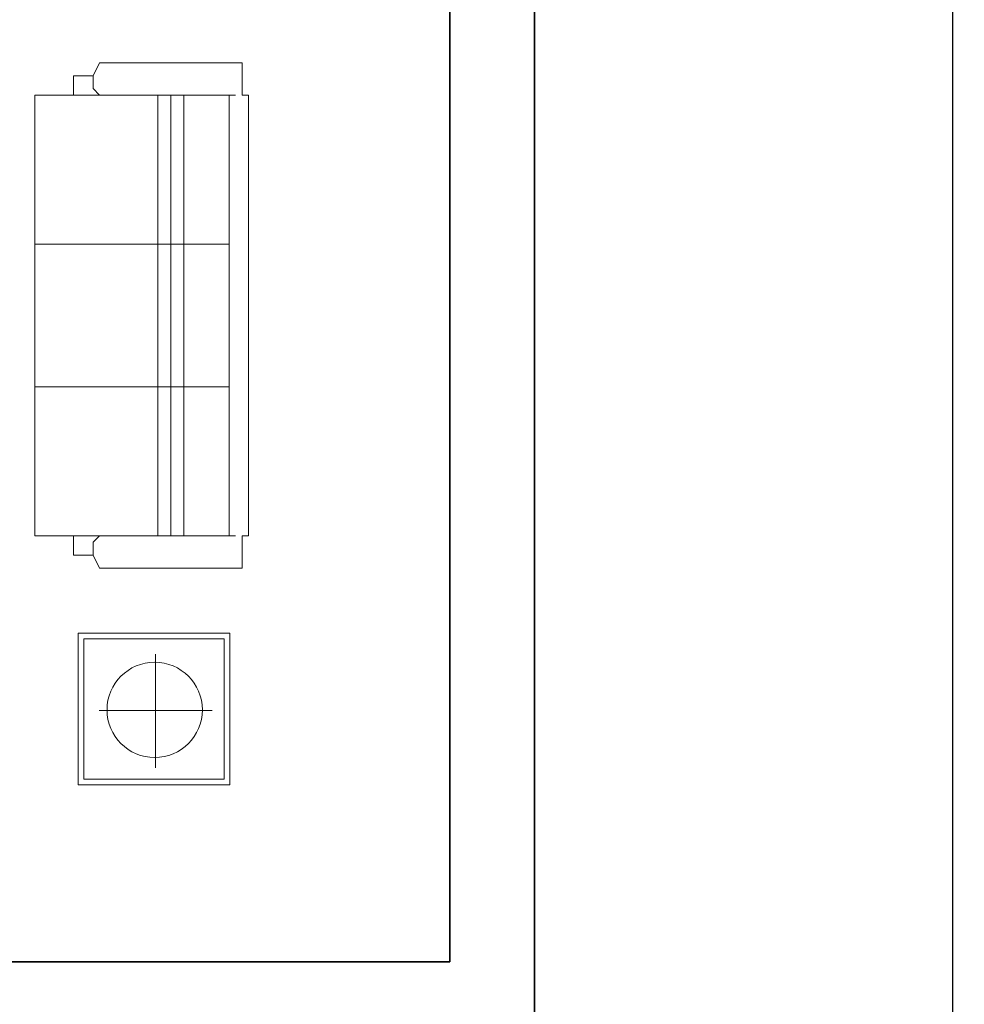
# Model space of a CAD drawing. Units: inches. Extents: x 1265 to 2734, y 1741 to 2595.
# Tile 6 of 10: x 2634 to 2734, y 1988 to 2092. Entities that reach past the tile are written whole.
import ezdxf

# ---------------------------------------------------------------- set-up
doc = ezdxf.new("R2010")
doc.units = ezdxf.units.IN
doc.header["$LTSCALE"] = 0.1
for name, color, linetype, lineweight in [('A-ANNO-DIMS', 2, 'Continuous', 18), ('A-WALL', 7, 'Continuous', 35), ('C-PROP', 7, 'Continuous', 35), ('Furniture', 8, 'Continuous', 15)]:
    doc.layers.add(name, color=color, linetype=linetype, lineweight=lineweight)
doc.styles.get("Standard").update_dxf_attribs({"font": 'arial.ttf', "height": 5})
doc.dimstyles.new('ISO-25', dxfattribs={"dimtxt": 5, "dimasz": 2.5, "dimexe": 1.25, "dimexo": 0.625, "dimtad": 1, "dimlunit": 3, "dimtxsty": 'Standard', "dimcen": 2.5, "dimadec": 0, "dimazin": 0, "dimtfac": 1, "dimtmove": 0, "dimatfit": 3, "dimfxl": 1, "dimarcsym": 0})

# ---------------------------------------------------------------- blocks, each defined once
blk = doc.blocks.new('*D3')
at = {"layer": 'A-ANNO-DIMS', "color": 0, "lineweight": -2, "transparency": 16777216}
for p, q in [((2689.23, 2542.66), (2734.23, 2542.66)), ((2732.98, 2540.16), (2732.98, 1789.16)), ((2689.23, 1786.66), (2734.23, 1786.66))]:
    blk.add_line(p, q, dxfattribs=at)
at = {"layer": 'A-ANNO-DIMS', "color": 0, "lineweight": 100, "transparency": 16777216}
for points in [[(2732.56, 2540.16), (2733.39, 2540.16), (2732.98, 2542.66)], [(2732.56, 1789.16), (2733.39, 1789.16), (2732.98, 1786.66)]]:
    blk.add_solid(points, dxfattribs=at)
at = {"layer": 'Defpoints', "color": 0, "lineweight": 100, "transparency": 16777216}
for p in [(2688.6, 2542.66), (2688.6, 1786.66), (2732.98, 1786.66)]:
    blk.add_point(p, dxfattribs=at)
at = {"layer": 'A-ANNO-DIMS', "color": 0, "transparency": 16777216, "insert": (2729.8, 2164.66), "char_height": 5, "attachment_point": 5, "rotation": 90}
blk.add_mtext("63'", dxfattribs=at)
blk = doc.blocks.new('END-TABLE-ROUND-LAMP')
for p, q in [((0, 0), (0, 16.08)), ((0, 16.08), (16.08, 16.08)), ((16.08, 16.08), (16.08, 0)), ((0.58, 0.59), (0.58, 15.5)), ((0.58, 15.5), (15.49, 15.5)), ((15.49, 15.5), (15.49, 0.59)), ((8.18, 13.85), (8.18, 1.8)), ((14.2, 7.89), (2.22, 7.89)), ((16.08, 0), (0, 0)), ((15.49, 0.59), (0.58, 0.59))]:
    blk.add_line(p, q)
blk.add_circle((8.11, 7.95), 5.06)

msp = doc.modelspace()

# ---------------------------------------------------------------- linework, layer by layer
at = {"layer": 'A-WALL'}
for p in [(2679.602, 2220.157), (2514.602, 1992.157)]:
    msp.add_line(p, (2679.602, 1992.157), dxfattribs=at)
at = {"layer": 'C-PROP'}
msp.add_line((2688.602, 2542.657), (2688.602, 1786.657), dxfattribs=at)
at = {"layer": 'Furniture'}
for p, q in [((2641.741, 2086.231), (2642.429, 2087.607)), ((2642.429, 2087.607), (2657.562, 2087.607)), ((2657.562, 2087.607), (2657.562, 2084.167)), ((2639.678, 2084.167), (2639.678, 2086.231)), ((2639.678, 2086.231), (2641.741, 2086.231)), ((2641.741, 2086.231), (2641.741, 2084.855)), ((2635.55, 2037.391), (2635.55, 2084.167)), ((2635.55, 2084.167), (2639.678, 2084.167)), ((2639.678, 2084.167), (2642.429, 2084.167)), ((2641.741, 2084.855), (2642.429, 2084.167)), ((2642.429, 2084.167), (2656.875, 2084.167)), ((2648.62, 2037.391), (2648.62, 2084.167)), ((2649.996, 2037.391), (2649.996, 2084.167)), ((2651.372, 2037.391), (2651.372, 2084.167)), ((2656.187, 2084.167), (2656.187, 2037.391)), ((2657.562, 2084.167), (2658.25, 2084.167)), ((2658.25, 2084.167), (2658.25, 2037.391)), ((2635.55, 2068.346), (2656.187, 2068.346)), ((2635.55, 2053.212), (2656.187, 2053.212)), ((2639.678, 2037.391), (2635.55, 2037.391)), ((2639.678, 2037.391), (2642.429, 2037.391)), ((2639.678, 2035.328), (2639.678, 2037.391)), ((2641.741, 2036.703), (2642.429, 2037.391)), ((2642.429, 2037.391), (2656.875, 2037.391)), ((2658.25, 2037.391), (2657.562, 2037.391)), ((2657.562, 2037.391), (2657.562, 2033.952)), ((2641.741, 2035.328), (2641.741, 2036.703)), ((2641.741, 2035.328), (2639.678, 2035.328)), ((2642.429, 2033.952), (2641.741, 2035.328)), ((2657.562, 2033.952), (2642.429, 2033.952))]:
    msp.add_line(p, q, dxfattribs=at)

# ---------------------------------------------------------------- block references
msp.add_blockref('END-TABLE-ROUND-LAMP', (2640.17, 2010.962), dxfattribs=at)

# ---------------------------------------------------------------- dimensions: what is measured, and where the dimension line sits
at = {"layer": 'A-ANNO-DIMS'}
dim = msp.add_linear_dim(base=(2732.978, 1786.657), p1=(2688.602, 2542.657), p2=(2688.602, 1786.657), angle=90, dimstyle='ISO-25', override={"dimclrd": 0, "dimclre": 0, "dimclrt": 0}, dxfattribs=at)
dim.commit()
dim.dimension.update_dxf_attribs({"geometry": '*D3', "text_midpoint": (2729.798, 2164.657)})

doc.saveas('drawing.dxf')
